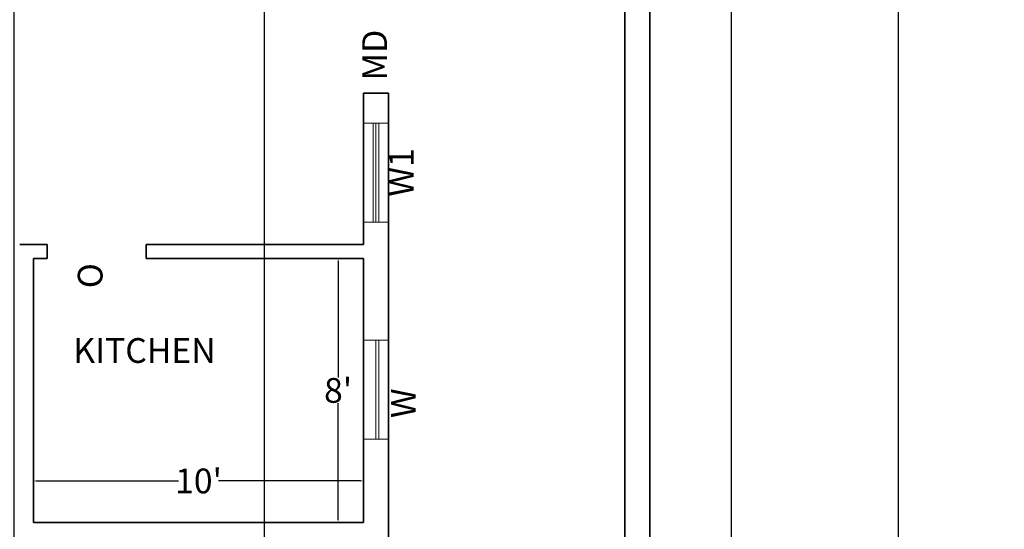
# Model space of a CAD drawing. Units: inches. Extents: x -2189 to 546, y 945 to 2684.
# Tile 5 of 10: x -492 to -134, y 2082 to 2267. Entities that reach past the tile are written whole.
import ezdxf

# ---------------------------------------------------------------- set-up
doc = ezdxf.new("R2010")
doc.units = ezdxf.units.IN
doc.header["$MEASUREMENT"] = 0
for name, color, linetype, lineweight in [('A-ANNO-DIMS', 2, 'Continuous', 13), ('A-ANNO-TEXT', 7, 'Continuous', 18), ('A-AREA-IDEN', 3, 'Continuous', 18), ('A-GLAZ', 4, 'Continuous', 18), ('A-WALL', 7, 'Continuous', 35)]:
    doc.layers.add(name, color=color, linetype=linetype, lineweight=lineweight)
doc.styles.get("Standard").update_dxf_attribs({"font": 'arial.ttf'})
doc.dimstyles.get("Standard").update_dxf_attribs({"dimtxt": 1, "dimasz": 1, "dimexe": 0.18, "dimexo": 0.0625, "dimgap": 0.09, "dimtad": 0, "dimtih": 1, "dimtoh": 1, "dimdec": 0, "dimzin": 0, "dimdsep": 46, "dimlunit": 3, "dimtxsty": 'Standard', "dimcen": 0.09, "dimadec": 0, "dimazin": 0, "dimtfac": 1, "dimtdec": 0, "dimtofl": 0, "dimtmove": 0, "dimatfit": 3, "dimfxl": 1, "dimtolj": 1, "dimtzin": 0, "dimarcsym": 0})

# ---------------------------------------------------------------- blocks, each defined once
blk = doc.blocks.new('*D59')
at = {"layer": 'A-ANNO-DIMS', "color": 0, "lineweight": -2, "transparency": 16777216}
for p, q in [((-486.78, 2084.24), (-486.78, 2099.44)), ((-485.78, 2099.26), (-434.08, 2099.26)), ((-367.78, 2099.26), (-419.48, 2099.26)), ((-366.78, 2084.24), (-366.78, 2099.44))]:
    blk.add_line(p, q, dxfattribs=at)
at = {"layer": 'A-ANNO-DIMS', "color": 0, "transparency": 16777216}
for points in [[(-485.78, 2099.43), (-485.78, 2099.09), (-486.78, 2099.26)], [(-367.78, 2099.43), (-367.78, 2099.09), (-366.78, 2099.26)]]:
    blk.add_solid(points, dxfattribs=at)
at = {"layer": 'Defpoints', "color": 0, "transparency": 16777216}
for p in [(-486.78, 2099.26), (-486.78, 2084.17), (-366.78, 2084.17)]:
    blk.add_point(p, dxfattribs=at)
at = {"layer": 'A-ANNO-DIMS', "color": 0, "transparency": 16777216, "insert": (-426.78, 2099.26), "char_height": 1, "attachment_point": 5}
blk.add_mtext("\\A1;{\\H9x;10'}", dxfattribs=at)
blk = doc.blocks.new('*D60')
at = {"layer": 'A-ANNO-DIMS', "color": 0, "lineweight": -2, "transparency": 16777216}
for p, q in [((-366.84, 2180.17), (-376.23, 2180.17)), ((-376.05, 2179.17), (-376.05, 2136.86)), ((-376.05, 2085.17), (-376.05, 2127.49)), ((-366.84, 2084.17), (-376.23, 2084.17))]:
    blk.add_line(p, q, dxfattribs=at)
at = {"layer": 'A-ANNO-DIMS', "color": 0, "transparency": 16777216}
for points in [[(-376.22, 2179.17), (-375.89, 2179.17), (-376.05, 2180.17)], [(-376.22, 2085.17), (-375.89, 2085.17), (-376.05, 2084.17)]]:
    blk.add_solid(points, dxfattribs=at)
at = {"layer": 'Defpoints', "color": 0, "transparency": 16777216}
for p in [(-376.05, 2180.17), (-366.78, 2180.17), (-366.78, 2084.17)]:
    blk.add_point(p, dxfattribs=at)
at = {"layer": 'A-ANNO-DIMS', "color": 0, "transparency": 16777216, "insert": (-376.05, 2132.17), "char_height": 1, "attachment_point": 5}
blk.add_mtext("\\A1;{\\H9x;8'}", dxfattribs=at)
blk = doc.blocks.new('*D79')
at = {"layer": 'A-ANNO-DIMS', "color": 0, "lineweight": -2, "transparency": 16777216}
for p, q in [((-262.72, 2600.17), (-172.26, 2600.17)), ((-172.44, 2599.17), (-172.44, 1833.96)), ((-172.44, 1050.17), (-172.44, 1815.39)), ((-262.72, 1049.17), (-172.26, 1049.17))]:
    blk.add_line(p, q, dxfattribs=at)
at = {"layer": 'A-ANNO-DIMS', "color": 0, "transparency": 16777216}
for points in [[(-172.6, 2599.17), (-172.27, 2599.17), (-172.44, 2600.17)], [(-172.6, 1050.17), (-172.27, 1050.17), (-172.44, 1049.17)]]:
    blk.add_solid(points, dxfattribs=at)
at = {"layer": 'Defpoints', "color": 0, "transparency": 16777216}
for p in [(-262.78, 2600.17), (-172.44, 2600.17), (-262.78, 1049.17)]:
    blk.add_point(p, dxfattribs=at)
at = {"layer": 'A-ANNO-DIMS', "color": 0, "transparency": 16777216, "insert": (-172.44, 1824.67), "char_height": 1, "attachment_point": 5}
blk.add_mtext('\\A1;{\\H18x;129\'-3"}', dxfattribs=at)
blk = doc.blocks.new('*D80')
at = {"layer": 'A-ANNO-DIMS', "color": 0, "lineweight": -2, "transparency": 16777216}
for p, q in [((-271.72, 2591.17), (-233.01, 2591.17)), ((-233.19, 2590.17), (-233.19, 1833.95)), ((-233.19, 1059.17), (-233.19, 1815.39)), ((-271.72, 1058.17), (-233.01, 1058.17))]:
    blk.add_line(p, q, dxfattribs=at)
at = {"layer": 'A-ANNO-DIMS', "color": 0, "transparency": 16777216}
for points in [[(-233.36, 2590.17), (-233.03, 2590.17), (-233.19, 2591.17)], [(-233.36, 1059.17), (-233.03, 1059.17), (-233.19, 1058.17)]]:
    blk.add_solid(points, dxfattribs=at)
at = {"layer": 'Defpoints', "color": 0, "transparency": 16777216}
for p in [(-271.78, 2591.17), (-233.19, 2591.17), (-271.78, 1058.17)]:
    blk.add_point(p, dxfattribs=at)
at = {"layer": 'A-ANNO-DIMS', "color": 0, "transparency": 16777216, "insert": (-233.19, 1824.67), "char_height": 1, "attachment_point": 5}
blk.add_mtext('\\A1;{\\H18x;127\'-9"}', dxfattribs=at)
blk = doc.blocks.new('WIN-36X9')
for p, q in [((0, 5.5), (36, 5.5)), ((0, 5.5), (36, 5.5)), ((0, 4.5), (36, 4.5)), ((0, 3.5), (36, 3.5))]:
    blk.add_line(p, q)
blk.add_lwpolyline([(0, 0), (0, 9), (36, 9), (36, 0)], close=True)
blk = doc.blocks.new('WIN-36X9-TWINLINE')
for p, q in [((4.5, 0), (4.5, 36)), ((5.5, 0), (5.5, 36))]:
    blk.add_line(p, q)
blk.add_lwpolyline([(9, 0), (0, 0), (0, 36), (9, 36)], close=True)
blk = doc.blocks.new('*D104')
at = {"layer": 'A-ANNO-DIMS', "color": 0, "lineweight": -2, "transparency": 16777216}
for p, q in [((-493.78, 1873.24), (-493.78, 2683.65)), ((-492.78, 2683.47), (-449.69, 2683.47)), ((-403.78, 2683.47), (-446.86, 2683.47)), ((-402.78, 1873.24), (-402.78, 2683.65))]:
    blk.add_line(p, q, dxfattribs=at)
at = {"layer": 'A-ANNO-DIMS', "color": 0, "transparency": 16777216}
for points in [[(-492.78, 2683.64), (-492.78, 2683.31), (-493.78, 2683.47)], [(-403.78, 2683.64), (-403.78, 2683.31), (-402.78, 2683.47)]]:
    blk.add_solid(points, dxfattribs=at)
at = {"layer": 'Defpoints', "color": 0, "transparency": 16777216}
for p in [(-402.78, 2683.47), (-493.78, 1873.17), (-402.78, 1873.17)]:
    blk.add_point(p, dxfattribs=at)
at = {"layer": 'A-ANNO-DIMS', "color": 0, "transparency": 16777216, "insert": (-448.28, 2683.47), "char_height": 1, "attachment_point": 5}
blk.add_mtext('\\A1;7\'-7"', dxfattribs=at)

msp = doc.modelspace()

# ---------------------------------------------------------------- linework, layer by layer
at = {"layer": 'A-WALL'}
for p, q in [((-262.78, 2600.17), (-262.78, 1049.17)), ((-271.78, 2591.17), (-271.78, 1058.17)), ((-366.78, 2185.17), (-366.78, 2240.2)), ((-366.78, 2240.2), (-357.78, 2240.2)), ((-357.78, 2074.17), (-357.78, 2240.2)), ((-481.78, 2185.17), (-491.78, 2185.17)), ((-481.78, 2180.17), (-481.78, 2185.17)), ((-366.78, 2185.17), (-445.78, 2185.17)), ((-445.78, 2180.17), (-445.78, 2185.17)), ((-486.78, 2084.17), (-486.78, 2180.17)), ((-481.78, 2180.17), (-486.78, 2180.17)), ((-366.78, 2180.17), (-445.78, 2180.17)), ((-366.78, 2084.17), (-366.78, 2180.17)), ((-366.78, 2084.17), (-486.78, 2084.17))]:
    msp.add_line(p, q, dxfattribs=at)

# ---------------------------------------------------------------- block references
at = {"layer": 'A-GLAZ', "rotation": 90.00000000000111}
msp.add_blockref('WIN-36X9', (-357.78, 2193.33), dxfattribs=at)
at = {"layer": 'A-GLAZ'}
msp.add_blockref('WIN-36X9-TWINLINE', (-366.78, 2114.48), dxfattribs=at)

# ---------------------------------------------------------------- texts
at = {"layer": 'A-ANNO-TEXT', "char_height": 9, "attachment_point": 1, "rotation": 90}
for s, width, heights, insert in [('MD', 16.482, [0], (-367.28, 2244.87)), ('W1', 11.3125, [0], (-357.59, 2202.6)), ('O', 18.6541, [0.207], (-470.67, 2169.32)), ('W', 11.3125, [0], (-356.83, 2122.11))]:
    msp.add_mtext_dynamic_manual_height_columns(s, width=width, gutter_width=1, heights=heights, dxfattribs=dict(at, insert=insert))
at = {"layer": 'A-AREA-IDEN', "insert": (-472.3, 2151.17), "char_height": 9, "attachment_point": 1}
msp.add_mtext_dynamic_manual_height_columns('KITCHEN', width=69.371, gutter_width=1, heights=[0], dxfattribs=at)

# ---------------------------------------------------------------- dimensions: what is measured, and where the dimension line sits
at = {"layer": 'A-ANNO-DIMS'}
dim = msp.add_linear_dim(base=(-402.78, 2683.47), p1=(-493.78, 1873.17), p2=(-402.78, 1873.17), dimstyle='Standard', override={"dimdec": 1, "dimlfac": 1, "dimrnd": 0, "dimzin": 1, "dimdsep": 46, "dimlunit": 4, "dimfrac": 2}, dxfattribs=at)
dim.commit()
dim.dimension.update_dxf_attribs({"geometry": '*D104', "text_midpoint": (-448.28, 2683.47)})
for base, p1, p2, angle, text, picture, middle in [((-172.44, 2600.17), (-262.78, 1049.17), (-262.78, 2600.17), 90, '{\\H18x;<>}', '*D79', (-172.44, 1824.67)), ((-233.19, 2591.17), (-271.78, 1058.17), (-271.78, 2591.17), 90, '{\\H18x;<>}', '*D80', (-233.19, 1824.67)), ((-376.05, 2180.17), (-366.78, 2084.17), (-366.78, 2180.17), 90, '{\\H9x;<>}', '*D60', (-376.05, 2132.17)), ((-486.78, 2099.26), (-366.78, 2084.17), (-486.78, 2084.17), 180, '{\\H9x;<>}', '*D59', (-426.78, 2099.26))]:
    dim = msp.add_linear_dim(base=base, p1=p1, p2=p2, angle=angle, text=text, dimstyle='Standard', override={"dimclrd": 0, "dimclre": 0, "dimclrt": 0}, dxfattribs=at)
    dim.commit()
    dim.dimension.update_dxf_attribs({"geometry": picture, "text_midpoint": middle})

doc.saveas('drawing.dxf')
